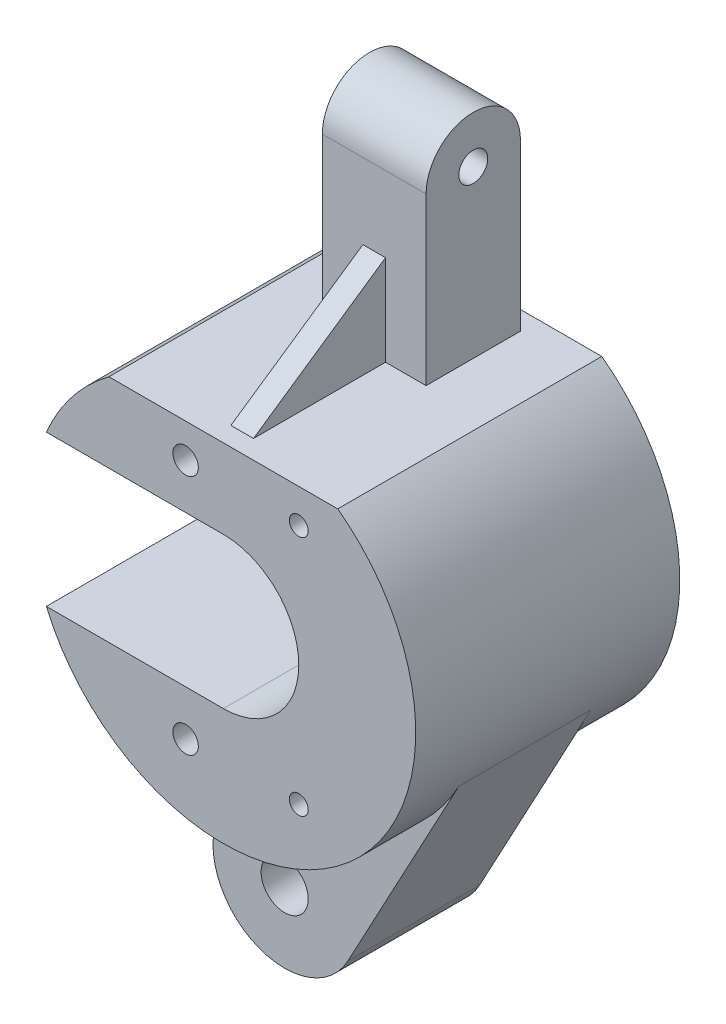
ISO-10303-21;
HEADER;
FILE_DESCRIPTION(('STEP AP214'),'2;1');
FILE_NAME('part.step','',(''),(''),'','','');
FILE_SCHEMA(('AUTOMOTIVE_DESIGN { 1 0 10303 214 1 1 1 1 }'));
ENDSEC;
DATA;
#1=APPLICATION_CONTEXT('core data for automotive mechanical design processes');
#2=APPLICATION_PROTOCOL_DEFINITION('international standard','automotive_design',2000,#1);
#3=PRODUCT_CONTEXT('',#1,'mechanical');
#4=PRODUCT('Part','Part','',(#3));
#5=PRODUCT_RELATED_PRODUCT_CATEGORY('part','',(#4));
#6=PRODUCT_DEFINITION_FORMATION('','',#4);
#7=PRODUCT_DEFINITION_CONTEXT('part definition',#1,'design');
#8=PRODUCT_DEFINITION('design','',#6,#7);
#9=PRODUCT_DEFINITION_SHAPE('','',#8);
#10=(LENGTH_UNIT() NAMED_UNIT(*) SI_UNIT(.MILLI.,.METRE.));
#11=(NAMED_UNIT(*) PLANE_ANGLE_UNIT() SI_UNIT($,.RADIAN.));
#12=(NAMED_UNIT(*) SI_UNIT($,.STERADIAN.) SOLID_ANGLE_UNIT());
#13=UNCERTAINTY_MEASURE_WITH_UNIT(LENGTH_MEASURE(1.E-05),#10,'distance_accuracy_value','');
#14=(GEOMETRIC_REPRESENTATION_CONTEXT(3) GLOBAL_UNCERTAINTY_ASSIGNED_CONTEXT((#13)) GLOBAL_UNIT_ASSIGNED_CONTEXT((#10,
#11,#12)) REPRESENTATION_CONTEXT('',''));
#15=CARTESIAN_POINT('',(0.,0.,0.));
#16=DIRECTION('',(0.,0.,1.));
#17=DIRECTION('',(1.,0.,0.));
#18=AXIS2_PLACEMENT_3D('',#15,#16,#17);
#19=CARTESIAN_POINT('',(0.,0.,70.));
#20=DIRECTION('',(0.,0.,1.));
#21=DIRECTION('',(1.,0.,0.));
#22=AXIS2_PLACEMENT_3D('',#19,#20,#21);
#23=PLANE('',#22);
#24=CARTESIAN_POINT('',(39.9916385221974,-64.,70.));
#25=DIRECTION('',(0.,0.,1.));
#26=DIRECTION('',(-1.,0.,0.));
#27=AXIS2_PLACEMENT_3D('',#24,#25,#26);
#28=CIRCLE('',#27,5.);
#29=CARTESIAN_POINT('',(34.9916385221974,-64.,70.));
#30=VERTEX_POINT('',#29);
#31=EDGE_CURVE('E274',#30,#30,#28,.T.);
#32=ORIENTED_EDGE('',*,*,#31,.F.);
#33=EDGE_LOOP('',(#32));
#34=FACE_BOUND('',#33,.T.);
#35=CARTESIAN_POINT('',(39.9916385221974,64.,70.));
#36=DIRECTION('',(0.,0.,1.));
#37=DIRECTION('',(1.,0.,0.));
#38=AXIS2_PLACEMENT_3D('',#35,#36,#37);
#39=CIRCLE('',#38,5.);
#40=CARTESIAN_POINT('',(44.9916385221974,64.,70.));
#41=VERTEX_POINT('',#40);
#42=EDGE_CURVE('E284',#41,#41,#39,.T.);
#43=ORIENTED_EDGE('',*,*,#42,.F.);
#44=EDGE_LOOP('',(#43));
#45=FACE_BOUND('',#44,.T.);
#46=CARTESIAN_POINT('',(0.,0.,70.));
#47=DIRECTION('',(0.,0.,1.));
#48=DIRECTION('',(1.,0.,0.));
#49=AXIS2_PLACEMENT_3D('',#46,#47,#48);
#50=CIRCLE('',#49,102.);
#51=CARTESIAN_POINT('',(-93.8296328459192,-40.,70.));
#52=VERTEX_POINT('',#51);
#53=CARTESIAN_POINT('',(60.6630035524124,82.,70.));
#54=VERTEX_POINT('',#53);
#55=EDGE_CURVE('E289',#52,#54,#50,.T.);
#56=ORIENTED_EDGE('',*,*,#55,.T.);
#57=DIRECTION('',(-1.,0.,0.));
#58=VECTOR('',#57,1.);
#59=CARTESIAN_POINT('',(-60.6630035524124,82.,70.));
#60=LINE('',#59,#58);
#61=CARTESIAN_POINT('',(-60.6630035524124,82.,70.));
#62=VERTEX_POINT('',#61);
#63=EDGE_CURVE('E291',#54,#62,#60,.T.);
#64=ORIENTED_EDGE('',*,*,#63,.T.);
#65=CARTESIAN_POINT('',(0.,0.,70.));
#66=DIRECTION('',(0.,0.,1.));
#67=DIRECTION('',(1.,0.,0.));
#68=AXIS2_PLACEMENT_3D('',#65,#66,#67);
#69=CIRCLE('',#68,102.);
#70=CARTESIAN_POINT('',(-93.8296328459192,40.,70.));
#71=VERTEX_POINT('',#70);
#72=EDGE_CURVE('E297',#62,#71,#69,.T.);
#73=ORIENTED_EDGE('',*,*,#72,.T.);
#74=DIRECTION('',(1.,0.,0.));
#75=VECTOR('',#74,1.);
#76=CARTESIAN_POINT('',(0.,40.,70.));
#77=LINE('',#76,#75);
#78=CARTESIAN_POINT('',(0.,40.,70.));
#79=VERTEX_POINT('',#78);
#80=EDGE_CURVE('E298',#71,#79,#77,.T.);
#81=ORIENTED_EDGE('',*,*,#80,.T.);
#82=CARTESIAN_POINT('',(0.,0.,70.));
#83=DIRECTION('',(0.,0.,-1.));
#84=DIRECTION('',(1.,0.,0.));
#85=AXIS2_PLACEMENT_3D('',#82,#83,#84);
#86=CIRCLE('',#85,40.);
#87=CARTESIAN_POINT('',(0.,-40.,70.));
#88=VERTEX_POINT('',#87);
#89=EDGE_CURVE('E296',#79,#88,#86,.T.);
#90=ORIENTED_EDGE('',*,*,#89,.T.);
#91=DIRECTION('',(-1.,0.,0.));
#92=VECTOR('',#91,1.);
#93=CARTESIAN_POINT('',(0.,-40.,70.));
#94=LINE('',#93,#92);
#95=EDGE_CURVE('E305',#88,#52,#94,.T.);
#96=ORIENTED_EDGE('',*,*,#95,.T.);
#97=EDGE_LOOP('',(#56,#64,#73,#81,#90,#96));
#98=FACE_BOUND('',#97,.T.);
#99=CARTESIAN_POINT('',(-20.,64.,70.));
#100=DIRECTION('',(0.,0.,1.));
#101=DIRECTION('',(1.,0.,0.));
#102=AXIS2_PLACEMENT_3D('',#99,#100,#101);
#103=CIRCLE('',#102,6.75);
#104=CARTESIAN_POINT('',(-13.25,64.,70.));
#105=VERTEX_POINT('',#104);
#106=EDGE_CURVE('E282',#105,#105,#103,.T.);
#107=ORIENTED_EDGE('',*,*,#106,.F.);
#108=EDGE_LOOP('',(#107));
#109=FACE_BOUND('',#108,.T.);
#110=CARTESIAN_POINT('',(-20.,-64.,70.));
#111=DIRECTION('',(0.,0.,1.));
#112=DIRECTION('',(-1.,0.,0.));
#113=AXIS2_PLACEMENT_3D('',#110,#111,#112);
#114=CIRCLE('',#113,6.75);
#115=CARTESIAN_POINT('',(-26.75,-64.,70.));
#116=VERTEX_POINT('',#115);
#117=EDGE_CURVE('E275',#116,#116,#114,.T.);
#118=ORIENTED_EDGE('',*,*,#117,.F.);
#119=EDGE_LOOP('',(#118));
#120=FACE_BOUND('',#119,.T.);
#121=ADVANCED_FACE('F43',(#34,#45,#98,#109,#120),#23,.T.);
#122=CARTESIAN_POINT('',(0.,0.,-70.));
#123=DIRECTION('',(0.,0.,1.));
#124=DIRECTION('',(1.,0.,0.));
#125=AXIS2_PLACEMENT_3D('',#122,#123,#124);
#126=PLANE('',#125);
#127=CARTESIAN_POINT('',(39.9916385221974,-64.,-70.));
#128=DIRECTION('',(0.,0.,1.));
#129=DIRECTION('',(1.,0.,0.));
#130=AXIS2_PLACEMENT_3D('',#127,#128,#129);
#131=CIRCLE('',#130,7.00000000000006);
#132=CARTESIAN_POINT('',(46.9916385221974,-64.,-70.));
#133=VERTEX_POINT('',#132);
#134=EDGE_CURVE('E337',#133,#133,#131,.T.);
#135=ORIENTED_EDGE('',*,*,#134,.T.);
#136=EDGE_LOOP('',(#135));
#137=FACE_BOUND('',#136,.T.);
#138=CARTESIAN_POINT('',(39.9916385221974,64.,-70.));
#139=DIRECTION('',(0.,0.,1.));
#140=DIRECTION('',(1.,0.,0.));
#141=AXIS2_PLACEMENT_3D('',#138,#139,#140);
#142=CIRCLE('',#141,7.00000000000006);
#143=CARTESIAN_POINT('',(46.9916385221974,64.,-70.));
#144=VERTEX_POINT('',#143);
#145=EDGE_CURVE('E334',#144,#144,#142,.T.);
#146=ORIENTED_EDGE('',*,*,#145,.T.);
#147=EDGE_LOOP('',(#146));
#148=FACE_BOUND('',#147,.T.);
#149=CARTESIAN_POINT('',(0.,0.,-70.));
#150=DIRECTION('',(0.,0.,1.));
#151=DIRECTION('',(1.,0.,0.));
#152=AXIS2_PLACEMENT_3D('',#149,#150,#151);
#153=CIRCLE('',#152,102.);
#154=CARTESIAN_POINT('',(-93.8296328459192,-40.,-70.));
#155=VERTEX_POINT('',#154);
#156=CARTESIAN_POINT('',(60.6630035524124,82.,-70.));
#157=VERTEX_POINT('',#156);
#158=EDGE_CURVE('E287',#155,#157,#153,.T.);
#159=ORIENTED_EDGE('',*,*,#158,.F.);
#160=DIRECTION('',(-1.,0.,0.));
#161=VECTOR('',#160,1.);
#162=CARTESIAN_POINT('',(0.,-40.,-70.));
#163=LINE('',#162,#161);
#164=CARTESIAN_POINT('',(0.,-40.,-70.));
#165=VERTEX_POINT('',#164);
#166=EDGE_CURVE('E294',#165,#155,#163,.T.);
#167=ORIENTED_EDGE('',*,*,#166,.F.);
#168=CARTESIAN_POINT('',(0.,0.,-70.));
#169=DIRECTION('',(0.,0.,-1.));
#170=DIRECTION('',(1.,0.,0.));
#171=AXIS2_PLACEMENT_3D('',#168,#169,#170);
#172=CIRCLE('',#171,40.);
#173=CARTESIAN_POINT('',(0.,40.,-70.));
#174=VERTEX_POINT('',#173);
#175=EDGE_CURVE('E311',#174,#165,#172,.T.);
#176=ORIENTED_EDGE('',*,*,#175,.F.);
#177=DIRECTION('',(1.,0.,0.));
#178=VECTOR('',#177,1.);
#179=CARTESIAN_POINT('',(0.,40.,-70.));
#180=LINE('',#179,#178);
#181=CARTESIAN_POINT('',(-93.8296328459192,40.,-70.));
#182=VERTEX_POINT('',#181);
#183=EDGE_CURVE('E313',#182,#174,#180,.T.);
#184=ORIENTED_EDGE('',*,*,#183,.F.);
#185=CARTESIAN_POINT('',(0.,0.,-70.));
#186=DIRECTION('',(0.,0.,1.));
#187=DIRECTION('',(1.,0.,0.));
#188=AXIS2_PLACEMENT_3D('',#185,#186,#187);
#189=CIRCLE('',#188,102.);
#190=CARTESIAN_POINT('',(-60.6630035524124,82.,-70.));
#191=VERTEX_POINT('',#190);
#192=EDGE_CURVE('E310',#191,#182,#189,.T.);
#193=ORIENTED_EDGE('',*,*,#192,.F.);
#194=DIRECTION('',(-1.,0.,0.));
#195=VECTOR('',#194,1.);
#196=CARTESIAN_POINT('',(-60.6630035524124,82.,-70.));
#197=LINE('',#196,#195);
#198=EDGE_CURVE('E307',#157,#191,#197,.T.);
#199=ORIENTED_EDGE('',*,*,#198,.F.);
#200=EDGE_LOOP('',(#159,#167,#176,#184,#193,#199));
#201=FACE_BOUND('',#200,.T.);
#202=CARTESIAN_POINT('',(-20.,64.,-70.));
#203=DIRECTION('',(0.,0.,1.));
#204=DIRECTION('',(1.,0.,0.));
#205=AXIS2_PLACEMENT_3D('',#202,#203,#204);
#206=CIRCLE('',#205,6.75);
#207=CARTESIAN_POINT('',(-13.25,64.,-70.));
#208=VERTEX_POINT('',#207);
#209=EDGE_CURVE('E278',#208,#208,#206,.T.);
#210=ORIENTED_EDGE('',*,*,#209,.T.);
#211=EDGE_LOOP('',(#210));
#212=FACE_BOUND('',#211,.T.);
#213=CARTESIAN_POINT('',(-20.,-64.,-70.));
#214=DIRECTION('',(0.,0.,1.));
#215=DIRECTION('',(-1.,0.,0.));
#216=AXIS2_PLACEMENT_3D('',#213,#214,#215);
#217=CIRCLE('',#216,6.75);
#218=CARTESIAN_POINT('',(-26.75,-64.,-70.));
#219=VERTEX_POINT('',#218);
#220=EDGE_CURVE('E271',#219,#219,#217,.T.);
#221=ORIENTED_EDGE('',*,*,#220,.T.);
#222=EDGE_LOOP('',(#221));
#223=FACE_BOUND('',#222,.T.);
#224=ADVANCED_FACE('F348',(#137,#148,#201,#212,#223),#126,.F.);
#225=CARTESIAN_POINT('',(0.,0.,70.));
#226=DIRECTION('',(0.,0.,-1.));
#227=DIRECTION('',(-1.,0.,0.));
#228=AXIS2_PLACEMENT_3D('',#225,#226,#227);
#229=CYLINDRICAL_SURFACE('',#228,102.);
#230=DIRECTION('',(0.,0.,-1.));
#231=VECTOR('',#230,1.);
#232=CARTESIAN_POINT('',(-27.5,-98.2229606558466,35.));
#233=LINE('',#232,#231);
#234=CARTESIAN_POINT('',(-27.5,-98.2229606558466,35.));
#235=VERTEX_POINT('',#234);
#236=CARTESIAN_POINT('',(-27.5,-98.2229606558466,-35.));
#237=VERTEX_POINT('',#236);
#238=EDGE_CURVE('E64',#235,#237,#233,.T.);
#239=ORIENTED_EDGE('',*,*,#238,.F.);
#240=CARTESIAN_POINT('',(0.,0.,35.));
#241=DIRECTION('',(0.,0.,1.));
#242=DIRECTION('',(1.,0.,0.));
#243=AXIS2_PLACEMENT_3D('',#240,#241,#242);
#244=CIRCLE('',#243,102.);
#245=CARTESIAN_POINT('',(-2.49082671878777,-101.969582632553,35.));
#246=VERTEX_POINT('',#245);
#247=EDGE_CURVE('E56',#235,#246,#244,.T.);
#248=ORIENTED_EDGE('',*,*,#247,.T.);
#249=DIRECTION('',(0.,0.,-1.));
#250=VECTOR('',#249,1.);
#251=CARTESIAN_POINT('',(-2.49082671878777,-101.969582632553,35.));
#252=LINE('',#251,#250);
#253=CARTESIAN_POINT('',(-2.49082671878777,-101.969582632553,-35.));
#254=VERTEX_POINT('',#253);
#255=EDGE_CURVE('E201',#246,#254,#252,.T.);
#256=ORIENTED_EDGE('',*,*,#255,.T.);
#257=CARTESIAN_POINT('',(0.,0.,-35.));
#258=DIRECTION('',(0.,0.,1.));
#259=DIRECTION('',(1.,0.,0.));
#260=AXIS2_PLACEMENT_3D('',#257,#258,#259);
#261=CIRCLE('',#260,102.);
#262=EDGE_CURVE('E705',#237,#254,#261,.T.);
#263=ORIENTED_EDGE('',*,*,#262,.F.);
#264=EDGE_LOOP('',(#239,#248,#256,#263));
#265=FACE_BOUND('',#264,.T.);
#266=DIRECTION('',(0.,0.,-1.));
#267=VECTOR('',#266,1.);
#268=CARTESIAN_POINT('',(-1.81474518083109,-101.983855094464,35.));
#269=LINE('',#268,#267);
#270=CARTESIAN_POINT('',(-1.81474518083109,-101.983855094464,35.));
#271=VERTEX_POINT('',#270);
#272=CARTESIAN_POINT('',(-1.81474518083109,-101.983855094464,-35.));
#273=VERTEX_POINT('',#272);
#274=EDGE_CURVE('E424',#271,#273,#269,.T.);
#275=ORIENTED_EDGE('',*,*,#274,.F.);
#276=CARTESIAN_POINT('',(89.8741576873943,-48.2352130707575,35.));
#277=VERTEX_POINT('',#276);
#278=EDGE_CURVE('E725',#271,#277,#244,.T.);
#279=ORIENTED_EDGE('',*,*,#278,.T.);
#280=DIRECTION('',(0.,0.,-1.));
#281=VECTOR('',#280,1.);
#282=CARTESIAN_POINT('',(89.8741576873943,-48.2352130707575,35.));
#283=LINE('',#282,#281);
#284=CARTESIAN_POINT('',(89.8741576873943,-48.2352130707575,-35.));
#285=VERTEX_POINT('',#284);
#286=EDGE_CURVE('E202',#277,#285,#283,.T.);
#287=ORIENTED_EDGE('',*,*,#286,.T.);
#288=EDGE_CURVE('E704',#273,#285,#261,.T.);
#289=ORIENTED_EDGE('',*,*,#288,.F.);
#290=EDGE_LOOP('',(#275,#279,#287,#289));
#291=FACE_BOUND('',#290,.T.);
#292=ORIENTED_EDGE('',*,*,#158,.T.);
#293=DIRECTION('',(0.,0.,-1.));
#294=VECTOR('',#293,1.);
#295=CARTESIAN_POINT('',(60.6630035524124,82.,70.));
#296=LINE('',#295,#294);
#297=EDGE_CURVE('E329',#54,#157,#296,.T.);
#298=ORIENTED_EDGE('',*,*,#297,.F.);
#299=ORIENTED_EDGE('',*,*,#55,.F.);
#300=DIRECTION('',(0.,0.,-1.));
#301=VECTOR('',#300,1.);
#302=CARTESIAN_POINT('',(-93.8296328459192,-40.,70.));
#303=LINE('',#302,#301);
#304=EDGE_CURVE('E302',#52,#155,#303,.T.);
#305=ORIENTED_EDGE('',*,*,#304,.T.);
#306=EDGE_LOOP('',(#292,#298,#299,#305));
#307=FACE_BOUND('',#306,.T.);
#308=ADVANCED_FACE('F353',(#265,#291,#307),#229,.T.);
#309=CARTESIAN_POINT('',(-60.6630035524124,82.,70.));
#310=DIRECTION('',(0.,-1.,0.));
#311=DIRECTION('',(0.,0.,-1.));
#312=AXIS2_PLACEMENT_3D('',#309,#310,#311);
#313=PLANE('',#312);
#314=DIRECTION('',(-1.,0.,0.));
#315=VECTOR('',#314,1.);
#316=CARTESIAN_POINT('',(27.5,82.,-10.));
#317=LINE('',#316,#315);
#318=CARTESIAN_POINT('',(27.5,82.,-10.));
#319=VERTEX_POINT('',#318);
#320=CARTESIAN_POINT('',(6.,82.,-10.));
#321=VERTEX_POINT('',#320);
#322=EDGE_CURVE('E268',#319,#321,#317,.T.);
#323=ORIENTED_EDGE('',*,*,#322,.T.);
#324=DIRECTION('',(0.,0.,-1.));
#325=VECTOR('',#324,1.);
#326=CARTESIAN_POINT('',(6.,82.,0.));
#327=LINE('',#326,#325);
#328=CARTESIAN_POINT('',(6.00000000000001,82.,60.));
#329=VERTEX_POINT('',#328);
#330=EDGE_CURVE('E220',#329,#321,#327,.T.);
#331=ORIENTED_EDGE('',*,*,#330,.F.);
#332=DIRECTION('',(-1.,0.,0.));
#333=VECTOR('',#332,1.);
#334=CARTESIAN_POINT('',(6.,82.,60.));
#335=LINE('',#334,#333);
#336=CARTESIAN_POINT('',(-6.,82.,60.));
#337=VERTEX_POINT('',#336);
#338=EDGE_CURVE('E219',#329,#337,#335,.T.);
#339=ORIENTED_EDGE('',*,*,#338,.T.);
#340=DIRECTION('',(0.,0.,-1.));
#341=VECTOR('',#340,1.);
#342=CARTESIAN_POINT('',(-6.,82.,0.));
#343=LINE('',#342,#341);
#344=CARTESIAN_POINT('',(-6.,82.,-10.));
#345=VERTEX_POINT('',#344);
#346=EDGE_CURVE('E212',#337,#345,#343,.T.);
#347=ORIENTED_EDGE('',*,*,#346,.T.);
#348=CARTESIAN_POINT('',(-27.5,82.,-10.));
#349=VERTEX_POINT('',#348);
#350=EDGE_CURVE('E270',#345,#349,#317,.T.);
#351=ORIENTED_EDGE('',*,*,#350,.T.);
#352=DIRECTION('',(0.,0.,-1.));
#353=VECTOR('',#352,1.);
#354=CARTESIAN_POINT('',(-27.5,82.,0.));
#355=LINE('',#354,#353);
#356=CARTESIAN_POINT('',(-27.5,82.,-60.));
#357=VERTEX_POINT('',#356);
#358=EDGE_CURVE('E253',#349,#357,#355,.T.);
#359=ORIENTED_EDGE('',*,*,#358,.T.);
#360=DIRECTION('',(-1.,0.,0.));
#361=VECTOR('',#360,1.);
#362=CARTESIAN_POINT('',(27.5,82.,-60.));
#363=LINE('',#362,#361);
#364=CARTESIAN_POINT('',(27.5,82.,-60.));
#365=VERTEX_POINT('',#364);
#366=EDGE_CURVE('E262',#365,#357,#363,.T.);
#367=ORIENTED_EDGE('',*,*,#366,.F.);
#368=DIRECTION('',(0.,0.,-1.));
#369=VECTOR('',#368,1.);
#370=CARTESIAN_POINT('',(27.5,82.,0.));
#371=LINE('',#370,#369);
#372=EDGE_CURVE('E237',#319,#365,#371,.T.);
#373=ORIENTED_EDGE('',*,*,#372,.F.);
#374=EDGE_LOOP('',(#323,#331,#339,#347,#351,#359,#367,#373));
#375=FACE_BOUND('',#374,.T.);
#376=ORIENTED_EDGE('',*,*,#198,.T.);
#377=DIRECTION('',(0.,0.,-1.));
#378=VECTOR('',#377,1.);
#379=CARTESIAN_POINT('',(-60.6630035524124,82.,70.));
#380=LINE('',#379,#378);
#381=EDGE_CURVE('E330',#62,#191,#380,.T.);
#382=ORIENTED_EDGE('',*,*,#381,.F.);
#383=ORIENTED_EDGE('',*,*,#63,.F.);
#384=ORIENTED_EDGE('',*,*,#297,.T.);
#385=EDGE_LOOP('',(#376,#382,#383,#384));
#386=FACE_BOUND('',#385,.T.);
#387=ADVANCED_FACE('F407',(#375,#386),#313,.F.);
#388=CARTESIAN_POINT('',(0.,0.,70.));
#389=DIRECTION('',(0.,0.,-1.));
#390=DIRECTION('',(-1.,0.,0.));
#391=AXIS2_PLACEMENT_3D('',#388,#389,#390);
#392=CYLINDRICAL_SURFACE('',#391,102.);
#393=ORIENTED_EDGE('',*,*,#192,.T.);
#394=DIRECTION('',(0.,0.,-1.));
#395=VECTOR('',#394,1.);
#396=CARTESIAN_POINT('',(-93.8296328459192,40.,70.));
#397=LINE('',#396,#395);
#398=EDGE_CURVE('E322',#71,#182,#397,.T.);
#399=ORIENTED_EDGE('',*,*,#398,.F.);
#400=ORIENTED_EDGE('',*,*,#72,.F.);
#401=ORIENTED_EDGE('',*,*,#381,.T.);
#402=EDGE_LOOP('',(#393,#399,#400,#401));
#403=FACE_BOUND('',#402,.T.);
#404=ADVANCED_FACE('F401',(#403),#392,.T.);
#405=CARTESIAN_POINT('',(0.,40.,70.));
#406=DIRECTION('',(0.,1.,0.));
#407=DIRECTION('',(-1.,0.,0.));
#408=AXIS2_PLACEMENT_3D('',#405,#406,#407);
#409=PLANE('',#408);
#410=ORIENTED_EDGE('',*,*,#183,.T.);
#411=DIRECTION('',(0.,0.,-1.));
#412=VECTOR('',#411,1.);
#413=CARTESIAN_POINT('',(0.,40.,70.));
#414=LINE('',#413,#412);
#415=EDGE_CURVE('E321',#79,#174,#414,.T.);
#416=ORIENTED_EDGE('',*,*,#415,.F.);
#417=ORIENTED_EDGE('',*,*,#80,.F.);
#418=ORIENTED_EDGE('',*,*,#398,.T.);
#419=EDGE_LOOP('',(#410,#416,#417,#418));
#420=FACE_BOUND('',#419,.T.);
#421=ADVANCED_FACE('F397',(#420),#409,.F.);
#422=CARTESIAN_POINT('',(0.,0.,70.));
#423=DIRECTION('',(0.,0.,-1.));
#424=DIRECTION('',(-1.,0.,0.));
#425=AXIS2_PLACEMENT_3D('',#422,#423,#424);
#426=CYLINDRICAL_SURFACE('',#425,40.);
#427=ORIENTED_EDGE('',*,*,#175,.T.);
#428=DIRECTION('',(0.,0.,-1.));
#429=VECTOR('',#428,1.);
#430=CARTESIAN_POINT('',(0.,-40.,70.));
#431=LINE('',#430,#429);
#432=EDGE_CURVE('E318',#88,#165,#431,.T.);
#433=ORIENTED_EDGE('',*,*,#432,.F.);
#434=ORIENTED_EDGE('',*,*,#89,.F.);
#435=ORIENTED_EDGE('',*,*,#415,.T.);
#436=EDGE_LOOP('',(#427,#433,#434,#435));
#437=FACE_BOUND('',#436,.T.);
#438=ADVANCED_FACE('F391',(#437),#426,.F.);
#439=CARTESIAN_POINT('',(0.,-40.,70.));
#440=DIRECTION('',(0.,-1.,0.));
#441=DIRECTION('',(1.,0.,0.));
#442=AXIS2_PLACEMENT_3D('',#439,#440,#441);
#443=PLANE('',#442);
#444=ORIENTED_EDGE('',*,*,#166,.T.);
#445=ORIENTED_EDGE('',*,*,#304,.F.);
#446=ORIENTED_EDGE('',*,*,#95,.F.);
#447=ORIENTED_EDGE('',*,*,#432,.T.);
#448=EDGE_LOOP('',(#444,#445,#446,#447));
#449=FACE_BOUND('',#448,.T.);
#450=ADVANCED_FACE('F395',(#449),#443,.F.);
#451=CARTESIAN_POINT('',(39.9916385221974,64.,70.));
#452=DIRECTION('',(0.,0.,-1.));
#453=DIRECTION('',(-1.,0.,0.));
#454=AXIS2_PLACEMENT_3D('',#451,#452,#453);
#455=CYLINDRICAL_SURFACE('',#454,5.);
#456=CARTESIAN_POINT('',(39.9916385221974,64.,-67.9999999999999));
#457=DIRECTION('',(0.,0.,1.));
#458=DIRECTION('',(1.,0.,0.));
#459=AXIS2_PLACEMENT_3D('',#456,#457,#458);
#460=CIRCLE('',#459,5.);
#461=CARTESIAN_POINT('',(44.9916385221974,64.,-67.9999999999999));
#462=VERTEX_POINT('',#461);
#463=EDGE_CURVE('E11',#462,#462,#460,.F.);
#464=ORIENTED_EDGE('',*,*,#463,.T.);
#465=EDGE_LOOP('',(#464));
#466=FACE_BOUND('',#465,.T.);
#467=ORIENTED_EDGE('',*,*,#42,.T.);
#468=EDGE_LOOP('',(#467));
#469=FACE_BOUND('',#468,.T.);
#470=ADVANCED_FACE('F386',(#466,#469),#455,.F.);
#471=CARTESIAN_POINT('',(-20.,64.,70.));
#472=DIRECTION('',(0.,0.,-1.));
#473=DIRECTION('',(-1.,0.,0.));
#474=AXIS2_PLACEMENT_3D('',#471,#472,#473);
#475=CYLINDRICAL_SURFACE('',#474,6.75);
#476=ORIENTED_EDGE('',*,*,#106,.T.);
#477=EDGE_LOOP('',(#476));
#478=FACE_BOUND('',#477,.T.);
#479=ORIENTED_EDGE('',*,*,#209,.F.);
#480=EDGE_LOOP('',(#479));
#481=FACE_BOUND('',#480,.T.);
#482=ADVANCED_FACE('F378',(#478,#481),#475,.F.);
#483=CARTESIAN_POINT('',(39.9916385221974,-64.,70.));
#484=DIRECTION('',(0.,0.,-1.));
#485=DIRECTION('',(-1.,0.,0.));
#486=AXIS2_PLACEMENT_3D('',#483,#484,#485);
#487=CYLINDRICAL_SURFACE('',#486,5.);
#488=CARTESIAN_POINT('',(39.9916385221974,-64.,-67.9999999999999));
#489=DIRECTION('',(0.,0.,1.));
#490=DIRECTION('',(1.,0.,0.));
#491=AXIS2_PLACEMENT_3D('',#488,#489,#490);
#492=CIRCLE('',#491,5.);
#493=CARTESIAN_POINT('',(44.9916385221974,-64.,-67.9999999999999));
#494=VERTEX_POINT('',#493);
#495=EDGE_CURVE('E55',#494,#494,#492,.F.);
#496=ORIENTED_EDGE('',*,*,#495,.T.);
#497=EDGE_LOOP('',(#496));
#498=FACE_BOUND('',#497,.T.);
#499=ORIENTED_EDGE('',*,*,#31,.T.);
#500=EDGE_LOOP('',(#499));
#501=FACE_BOUND('',#500,.T.);
#502=ADVANCED_FACE('F341',(#498,#501),#487,.F.);
#503=CARTESIAN_POINT('',(-20.,-64.,70.));
#504=DIRECTION('',(0.,0.,-1.));
#505=DIRECTION('',(-1.,0.,0.));
#506=AXIS2_PLACEMENT_3D('',#503,#504,#505);
#507=CYLINDRICAL_SURFACE('',#506,6.75);
#508=ORIENTED_EDGE('',*,*,#117,.T.);
#509=EDGE_LOOP('',(#508));
#510=FACE_BOUND('',#509,.T.);
#511=ORIENTED_EDGE('',*,*,#220,.F.);
#512=EDGE_LOOP('',(#511));
#513=FACE_BOUND('',#512,.T.);
#514=ADVANCED_FACE('F365',(#510,#513),#507,.F.);
#515=CARTESIAN_POINT('',(27.5,0.,-10.));
#516=DIRECTION('',(0.,0.,-1.));
#517=DIRECTION('',(-1.,0.,0.));
#518=AXIS2_PLACEMENT_3D('',#515,#516,#517);
#519=PLANE('',#518);
#520=DIRECTION('',(-1.,0.,0.));
#521=VECTOR('',#520,1.);
#522=CARTESIAN_POINT('',(6.,130.,-10.));
#523=LINE('',#522,#521);
#524=CARTESIAN_POINT('',(6.,130.,-10.));
#525=VERTEX_POINT('',#524);
#526=CARTESIAN_POINT('',(-6.,130.,-10.));
#527=VERTEX_POINT('',#526);
#528=EDGE_CURVE('E229',#525,#527,#523,.T.);
#529=ORIENTED_EDGE('',*,*,#528,.F.);
#530=DIRECTION('',(0.,-1.,0.));
#531=VECTOR('',#530,1.);
#532=CARTESIAN_POINT('',(6.,0.,-10.));
#533=LINE('',#532,#531);
#534=EDGE_CURVE('E211',#525,#321,#533,.T.);
#535=ORIENTED_EDGE('',*,*,#534,.T.);
#536=ORIENTED_EDGE('',*,*,#322,.F.);
#537=DIRECTION('',(0.,-1.,0.));
#538=VECTOR('',#537,1.);
#539=CARTESIAN_POINT('',(27.5,0.,-10.));
#540=LINE('',#539,#538);
#541=CARTESIAN_POINT('',(27.5,170.,-10.));
#542=VERTEX_POINT('',#541);
#543=EDGE_CURVE('E233',#542,#319,#540,.T.);
#544=ORIENTED_EDGE('',*,*,#543,.F.);
#545=DIRECTION('',(-1.,0.,0.));
#546=VECTOR('',#545,1.);
#547=CARTESIAN_POINT('',(27.5,170.,-10.));
#548=LINE('',#547,#546);
#549=CARTESIAN_POINT('',(-27.5,170.,-10.));
#550=VERTEX_POINT('',#549);
#551=EDGE_CURVE('E248',#542,#550,#548,.T.);
#552=ORIENTED_EDGE('',*,*,#551,.T.);
#553=DIRECTION('',(0.,-1.,0.));
#554=VECTOR('',#553,1.);
#555=CARTESIAN_POINT('',(-27.5,0.,-10.));
#556=LINE('',#555,#554);
#557=EDGE_CURVE('E235',#550,#349,#556,.T.);
#558=ORIENTED_EDGE('',*,*,#557,.T.);
#559=ORIENTED_EDGE('',*,*,#350,.F.);
#560=DIRECTION('',(0.,-1.,0.));
#561=VECTOR('',#560,1.);
#562=CARTESIAN_POINT('',(-6.,0.,-10.));
#563=LINE('',#562,#561);
#564=EDGE_CURVE('E209',#527,#345,#563,.T.);
#565=ORIENTED_EDGE('',*,*,#564,.F.);
#566=EDGE_LOOP('',(#529,#535,#536,#544,#552,#558,#559,#565));
#567=FACE_BOUND('',#566,.T.);
#568=ADVANCED_FACE('F368',(#567),#519,.F.);
#569=CARTESIAN_POINT('',(27.5,0.,-60.));
#570=DIRECTION('',(0.,0.,-1.));
#571=DIRECTION('',(-1.,0.,0.));
#572=AXIS2_PLACEMENT_3D('',#569,#570,#571);
#573=PLANE('',#572);
#574=DIRECTION('',(0.,-1.,0.));
#575=VECTOR('',#574,1.);
#576=CARTESIAN_POINT('',(-27.5,0.,-60.));
#577=LINE('',#576,#575);
#578=CARTESIAN_POINT('',(-27.5,170.,-60.));
#579=VERTEX_POINT('',#578);
#580=EDGE_CURVE('E251',#579,#357,#577,.T.);
#581=ORIENTED_EDGE('',*,*,#580,.F.);
#582=DIRECTION('',(-1.,0.,0.));
#583=VECTOR('',#582,1.);
#584=CARTESIAN_POINT('',(27.5,170.,-60.));
#585=LINE('',#584,#583);
#586=CARTESIAN_POINT('',(27.5,170.,-60.));
#587=VERTEX_POINT('',#586);
#588=EDGE_CURVE('E265',#587,#579,#585,.T.);
#589=ORIENTED_EDGE('',*,*,#588,.F.);
#590=DIRECTION('',(0.,-1.,0.));
#591=VECTOR('',#590,1.);
#592=CARTESIAN_POINT('',(27.5,0.,-60.));
#593=LINE('',#592,#591);
#594=EDGE_CURVE('E238',#587,#365,#593,.T.);
#595=ORIENTED_EDGE('',*,*,#594,.T.);
#596=ORIENTED_EDGE('',*,*,#366,.T.);
#597=EDGE_LOOP('',(#581,#589,#595,#596));
#598=FACE_BOUND('',#597,.T.);
#599=ADVANCED_FACE('F372',(#598),#573,.T.);
#600=CARTESIAN_POINT('',(27.5,170.,-35.));
#601=DIRECTION('',(-1.,0.,0.));
#602=DIRECTION('',(0.,0.,1.));
#603=AXIS2_PLACEMENT_3D('',#600,#601,#602);
#604=CYLINDRICAL_SURFACE('',#603,25.);
#605=CARTESIAN_POINT('',(-27.5,170.,-35.));
#606=DIRECTION('',(1.,0.,0.));
#607=DIRECTION('',(0.,0.,-1.));
#608=AXIS2_PLACEMENT_3D('',#605,#606,#607);
#609=CIRCLE('',#608,25.);
#610=EDGE_CURVE('E258',#579,#550,#609,.T.);
#611=ORIENTED_EDGE('',*,*,#610,.T.);
#612=ORIENTED_EDGE('',*,*,#551,.F.);
#613=CARTESIAN_POINT('',(27.5,170.,-35.));
#614=DIRECTION('',(1.,0.,0.));
#615=DIRECTION('',(0.,0.,-1.));
#616=AXIS2_PLACEMENT_3D('',#613,#614,#615);
#617=CIRCLE('',#616,25.);
#618=EDGE_CURVE('E243',#587,#542,#617,.T.);
#619=ORIENTED_EDGE('',*,*,#618,.F.);
#620=ORIENTED_EDGE('',*,*,#588,.T.);
#621=EDGE_LOOP('',(#611,#612,#619,#620));
#622=FACE_BOUND('',#621,.T.);
#623=ADVANCED_FACE('F497',(#622),#604,.T.);
#624=CARTESIAN_POINT('',(27.5,170.,-35.));
#625=DIRECTION('',(-1.,0.,0.));
#626=DIRECTION('',(0.,0.,1.));
#627=AXIS2_PLACEMENT_3D('',#624,#625,#626);
#628=CYLINDRICAL_SURFACE('',#627,7.66897657766724);
#629=CARTESIAN_POINT('',(27.5,170.,-35.));
#630=DIRECTION('',(1.,0.,0.));
#631=DIRECTION('',(0.,0.,-1.));
#632=AXIS2_PLACEMENT_3D('',#629,#630,#631);
#633=CIRCLE('',#632,7.66897657766724);
#634=CARTESIAN_POINT('',(27.5,170.,-42.6689765776672));
#635=VERTEX_POINT('',#634);
#636=EDGE_CURVE('E241',#635,#635,#633,.T.);
#637=ORIENTED_EDGE('',*,*,#636,.T.);
#638=EDGE_LOOP('',(#637));
#639=FACE_BOUND('',#638,.T.);
#640=CARTESIAN_POINT('',(-27.5,170.,-35.));
#641=DIRECTION('',(1.,0.,0.));
#642=DIRECTION('',(0.,0.,-1.));
#643=AXIS2_PLACEMENT_3D('',#640,#641,#642);
#644=CIRCLE('',#643,7.66897657766724);
#645=CARTESIAN_POINT('',(-27.5,170.,-42.6689765776672));
#646=VERTEX_POINT('',#645);
#647=EDGE_CURVE('E240',#646,#646,#644,.T.);
#648=ORIENTED_EDGE('',*,*,#647,.F.);
#649=EDGE_LOOP('',(#648));
#650=FACE_BOUND('',#649,.T.);
#651=ADVANCED_FACE('F506',(#639,#650),#628,.F.);
#652=CARTESIAN_POINT('',(27.5,0.,0.));
#653=DIRECTION('',(1.,0.,0.));
#654=DIRECTION('',(0.,0.,-1.));
#655=AXIS2_PLACEMENT_3D('',#652,#653,#654);
#656=PLANE('',#655);
#657=ORIENTED_EDGE('',*,*,#543,.T.);
#658=ORIENTED_EDGE('',*,*,#372,.T.);
#659=ORIENTED_EDGE('',*,*,#594,.F.);
#660=ORIENTED_EDGE('',*,*,#618,.T.);
#661=EDGE_LOOP('',(#657,#658,#659,#660));
#662=FACE_BOUND('',#661,.T.);
#663=ORIENTED_EDGE('',*,*,#636,.F.);
#664=EDGE_LOOP('',(#663));
#665=FACE_BOUND('',#664,.T.);
#666=ADVANCED_FACE('F517',(#662,#665),#656,.T.);
#667=CARTESIAN_POINT('',(-27.5,0.,0.));
#668=DIRECTION('',(1.,0.,0.));
#669=DIRECTION('',(0.,0.,-1.));
#670=AXIS2_PLACEMENT_3D('',#667,#668,#669);
#671=PLANE('',#670);
#672=ORIENTED_EDGE('',*,*,#557,.F.);
#673=ORIENTED_EDGE('',*,*,#610,.F.);
#674=ORIENTED_EDGE('',*,*,#580,.T.);
#675=ORIENTED_EDGE('',*,*,#358,.F.);
#676=EDGE_LOOP('',(#672,#673,#674,#675));
#677=FACE_BOUND('',#676,.T.);
#678=ORIENTED_EDGE('',*,*,#647,.T.);
#679=EDGE_LOOP('',(#678));
#680=FACE_BOUND('',#679,.T.);
#681=ADVANCED_FACE('F528',(#677,#680),#671,.F.);
#682=CARTESIAN_POINT('',(6.,83.7590227651305,57.434758467518));
#683=DIRECTION('',(0.,-0.824728851845978,-0.565528355551528));
#684=DIRECTION('',(0.,0.565528355551528,-0.824728851845978));
#685=AXIS2_PLACEMENT_3D('',#682,#683,#684);
#686=PLANE('',#685);
#687=DIRECTION('',(0.,-0.565528355551528,0.824728851845978));
#688=VECTOR('',#687,1.);
#689=CARTESIAN_POINT('',(-6.,83.7590227651305,57.434758467518));
#690=LINE('',#689,#688);
#691=EDGE_CURVE('E224',#527,#337,#690,.T.);
#692=ORIENTED_EDGE('',*,*,#691,.T.);
#693=ORIENTED_EDGE('',*,*,#338,.F.);
#694=DIRECTION('',(0.,-0.565528355551528,0.824728851845978));
#695=VECTOR('',#694,1.);
#696=CARTESIAN_POINT('',(6.,83.7590227651305,57.434758467518));
#697=LINE('',#696,#695);
#698=EDGE_CURVE('E213',#525,#329,#697,.T.);
#699=ORIENTED_EDGE('',*,*,#698,.F.);
#700=ORIENTED_EDGE('',*,*,#528,.T.);
#701=EDGE_LOOP('',(#692,#693,#699,#700));
#702=FACE_BOUND('',#701,.T.);
#703=ADVANCED_FACE('F536',(#702),#686,.F.);
#704=CARTESIAN_POINT('',(6.,0.,0.));
#705=DIRECTION('',(1.,0.,0.));
#706=DIRECTION('',(0.,0.,-1.));
#707=AXIS2_PLACEMENT_3D('',#704,#705,#706);
#708=PLANE('',#707);
#709=ORIENTED_EDGE('',*,*,#534,.F.);
#710=ORIENTED_EDGE('',*,*,#698,.T.);
#711=ORIENTED_EDGE('',*,*,#330,.T.);
#712=EDGE_LOOP('',(#709,#710,#711));
#713=FACE_BOUND('',#712,.T.);
#714=ADVANCED_FACE('F544',(#713),#708,.T.);
#715=CARTESIAN_POINT('',(-6.,0.,0.));
#716=DIRECTION('',(1.,0.,0.));
#717=DIRECTION('',(0.,0.,-1.));
#718=AXIS2_PLACEMENT_3D('',#715,#716,#717);
#719=PLANE('',#718);
#720=ORIENTED_EDGE('',*,*,#564,.T.);
#721=ORIENTED_EDGE('',*,*,#346,.F.);
#722=ORIENTED_EDGE('',*,*,#691,.F.);
#723=EDGE_LOOP('',(#720,#721,#722));
#724=FACE_BOUND('',#723,.T.);
#725=ADVANCED_FACE('F553',(#724),#719,.F.);
#726=CARTESIAN_POINT('',(-2.49082671878777,0.,35.));
#727=DIRECTION('',(1.,0.,0.));
#728=DIRECTION('',(0.,0.,-1.));
#729=AXIS2_PLACEMENT_3D('',#726,#727,#728);
#730=PLANE('',#729);
#731=DIRECTION('',(0.,-1.,0.));
#732=VECTOR('',#731,1.);
#733=CARTESIAN_POINT('',(-2.49082671878777,0.,-35.));
#734=LINE('',#733,#732);
#735=CARTESIAN_POINT('',(-2.49082671878776,-101.977840325735,-35.));
#736=VERTEX_POINT('',#735);
#737=EDGE_CURVE('E696',#254,#736,#734,.T.);
#738=ORIENTED_EDGE('',*,*,#737,.F.);
#739=ORIENTED_EDGE('',*,*,#255,.F.);
#740=DIRECTION('',(0.,-1.,0.));
#741=VECTOR('',#740,1.);
#742=CARTESIAN_POINT('',(-2.49082671878777,0.,35.));
#743=LINE('',#742,#741);
#744=CARTESIAN_POINT('',(-2.49082671878776,-101.977840325735,35.));
#745=VERTEX_POINT('',#744);
#746=EDGE_CURVE('E730',#246,#745,#743,.T.);
#747=ORIENTED_EDGE('',*,*,#746,.T.);
#748=DIRECTION('',(0.,0.,-1.));
#749=VECTOR('',#748,1.);
#750=CARTESIAN_POINT('',(-2.49082671878776,-101.977840325735,35.));
#751=LINE('',#750,#749);
#752=EDGE_CURVE('E720',#745,#736,#751,.T.);
#753=ORIENTED_EDGE('',*,*,#752,.T.);
#754=EDGE_LOOP('',(#738,#739,#747,#753));
#755=FACE_BOUND('',#754,.T.);
#756=ADVANCED_FACE('F562',(#755),#730,.T.);
#757=CARTESIAN_POINT('',(-27.5,0.,35.));
#758=DIRECTION('',(1.,0.,0.));
#759=DIRECTION('',(0.,0.,-1.));
#760=AXIS2_PLACEMENT_3D('',#757,#758,#759);
#761=PLANE('',#760);
#762=DIRECTION('',(0.,-1.,0.));
#763=VECTOR('',#762,1.);
#764=CARTESIAN_POINT('',(-27.5,0.,-35.));
#765=LINE('',#764,#763);
#766=CARTESIAN_POINT('',(-27.5,-111.367680385771,-35.));
#767=VERTEX_POINT('',#766);
#768=EDGE_CURVE('E203',#237,#767,#765,.T.);
#769=ORIENTED_EDGE('',*,*,#768,.T.);
#770=DIRECTION('',(0.,0.,-1.));
#771=VECTOR('',#770,1.);
#772=CARTESIAN_POINT('',(-27.5,-111.367680385771,35.));
#773=LINE('',#772,#771);
#774=CARTESIAN_POINT('',(-27.5,-111.367680385771,35.));
#775=VERTEX_POINT('',#774);
#776=EDGE_CURVE('E187',#775,#767,#773,.T.);
#777=ORIENTED_EDGE('',*,*,#776,.F.);
#778=DIRECTION('',(0.,-1.,0.));
#779=VECTOR('',#778,1.);
#780=CARTESIAN_POINT('',(-27.5,0.,35.));
#781=LINE('',#780,#779);
#782=EDGE_CURVE('E193',#235,#775,#781,.T.);
#783=ORIENTED_EDGE('',*,*,#782,.F.);
#784=ORIENTED_EDGE('',*,*,#238,.T.);
#785=EDGE_LOOP('',(#769,#777,#783,#784));
#786=FACE_BOUND('',#785,.T.);
#787=ADVANCED_FACE('F200',(#786),#761,.F.);
#788=CARTESIAN_POINT('',(-2.49082671878777,-139.977840325735,35.));
#789=DIRECTION('',(0.,0.,-1.));
#790=DIRECTION('',(-1.,0.,0.));
#791=AXIS2_PLACEMENT_3D('',#788,#789,#790);
#792=CYLINDRICAL_SURFACE('',#791,38.);
#793=CARTESIAN_POINT('',(-2.49082671878777,-139.977840325735,-35.));
#794=DIRECTION('',(0.,0.,1.));
#795=DIRECTION('',(1.,0.,0.));
#796=AXIS2_PLACEMENT_3D('',#793,#794,#795);
#797=CIRCLE('',#796,38.);
#798=CARTESIAN_POINT('',(30.9917026157317,-157.947821665821,-35.));
#799=VERTEX_POINT('',#798);
#800=EDGE_CURVE('E709',#767,#799,#797,.T.);
#801=ORIENTED_EDGE('',*,*,#800,.T.);
#802=DIRECTION('',(0.,0.,-1.));
#803=VECTOR('',#802,1.);
#804=CARTESIAN_POINT('',(30.9917026157317,-157.947821665821,35.));
#805=LINE('',#804,#803);
#806=CARTESIAN_POINT('',(30.9917026157317,-157.947821665821,35.));
#807=VERTEX_POINT('',#806);
#808=EDGE_CURVE('E189',#807,#799,#805,.T.);
#809=ORIENTED_EDGE('',*,*,#808,.F.);
#810=CARTESIAN_POINT('',(-2.49082671878777,-139.977840325735,35.));
#811=DIRECTION('',(0.,0.,1.));
#812=DIRECTION('',(1.,0.,0.));
#813=AXIS2_PLACEMENT_3D('',#810,#811,#812);
#814=CIRCLE('',#813,38.);
#815=EDGE_CURVE('E182',#775,#807,#814,.T.);
#816=ORIENTED_EDGE('',*,*,#815,.F.);
#817=ORIENTED_EDGE('',*,*,#776,.T.);
#818=EDGE_LOOP('',(#801,#809,#816,#817));
#819=FACE_BOUND('',#818,.T.);
#820=ADVANCED_FACE('F184',(#819),#792,.T.);
#821=CARTESIAN_POINT('',(89.8741576873943,-48.2352130707575,35.));
#822=DIRECTION('',(-0.88111919301367,0.472894245791741,0.));
#823=DIRECTION('',(-0.472894245791741,-0.88111919301367,0.));
#824=AXIS2_PLACEMENT_3D('',#821,#822,#823);
#825=PLANE('',#824);
#826=DIRECTION('',(0.472894245791741,0.88111919301367,0.));
#827=VECTOR('',#826,1.);
#828=CARTESIAN_POINT('',(89.8741576873943,-48.2352130707575,-35.));
#829=LINE('',#828,#827);
#830=EDGE_CURVE('E715',#799,#285,#829,.T.);
#831=ORIENTED_EDGE('',*,*,#830,.T.);
#832=ORIENTED_EDGE('',*,*,#286,.F.);
#833=DIRECTION('',(0.472894245791741,0.88111919301367,0.));
#834=VECTOR('',#833,1.);
#835=CARTESIAN_POINT('',(89.8741576873943,-48.2352130707575,35.));
#836=LINE('',#835,#834);
#837=EDGE_CURVE('E195',#807,#277,#836,.T.);
#838=ORIENTED_EDGE('',*,*,#837,.F.);
#839=ORIENTED_EDGE('',*,*,#808,.T.);
#840=EDGE_LOOP('',(#831,#832,#838,#839));
#841=FACE_BOUND('',#840,.T.);
#842=ADVANCED_FACE('F587',(#841),#825,.F.);
#843=CARTESIAN_POINT('',(-2.49082671878777,-139.977840325735,35.));
#844=DIRECTION('',(0.,0.,-1.));
#845=DIRECTION('',(-1.,0.,0.));
#846=AXIS2_PLACEMENT_3D('',#843,#844,#845);
#847=CYLINDRICAL_SURFACE('',#846,12.5);
#848=CARTESIAN_POINT('',(-2.49082671878777,-139.977840325735,35.));
#849=DIRECTION('',(0.,0.,1.));
#850=DIRECTION('',(1.,0.,0.));
#851=AXIS2_PLACEMENT_3D('',#848,#849,#850);
#852=CIRCLE('',#851,12.5);
#853=CARTESIAN_POINT('',(10.0091732812122,-139.977840325735,35.));
#854=VERTEX_POINT('',#853);
#855=EDGE_CURVE('E717',#854,#854,#852,.T.);
#856=ORIENTED_EDGE('',*,*,#855,.T.);
#857=EDGE_LOOP('',(#856));
#858=FACE_BOUND('',#857,.T.);
#859=CARTESIAN_POINT('',(-2.49082671878777,-139.977840325735,-35.));
#860=DIRECTION('',(0.,0.,1.));
#861=DIRECTION('',(1.,0.,0.));
#862=AXIS2_PLACEMENT_3D('',#859,#860,#861);
#863=CIRCLE('',#862,12.5);
#864=CARTESIAN_POINT('',(10.0091732812122,-139.977840325735,-35.));
#865=VERTEX_POINT('',#864);
#866=EDGE_CURVE('E691',#865,#865,#863,.T.);
#867=ORIENTED_EDGE('',*,*,#866,.F.);
#868=EDGE_LOOP('',(#867));
#869=FACE_BOUND('',#868,.T.);
#870=ADVANCED_FACE('F597',(#858,#869),#847,.F.);
#871=CARTESIAN_POINT('',(-2.49082671878777,-139.977840325735,35.));
#872=DIRECTION('',(0.,0.,-1.));
#873=DIRECTION('',(-1.,0.,0.));
#874=AXIS2_PLACEMENT_3D('',#871,#872,#873);
#875=CYLINDRICAL_SURFACE('',#874,38.);
#876=CARTESIAN_POINT('',(-2.49082671878777,-139.977840325735,-35.));
#877=DIRECTION('',(0.,0.,1.));
#878=DIRECTION('',(1.,0.,0.));
#879=AXIS2_PLACEMENT_3D('',#876,#877,#878);
#880=CIRCLE('',#879,38.);
#881=EDGE_CURVE('E701',#273,#736,#880,.T.);
#882=ORIENTED_EDGE('',*,*,#881,.T.);
#883=ORIENTED_EDGE('',*,*,#752,.F.);
#884=CARTESIAN_POINT('',(-2.49082671878777,-139.977840325735,35.));
#885=DIRECTION('',(0.,0.,1.));
#886=DIRECTION('',(1.,0.,0.));
#887=AXIS2_PLACEMENT_3D('',#884,#885,#886);
#888=CIRCLE('',#887,38.);
#889=EDGE_CURVE('E716',#271,#745,#888,.T.);
#890=ORIENTED_EDGE('',*,*,#889,.F.);
#891=ORIENTED_EDGE('',*,*,#274,.T.);
#892=EDGE_LOOP('',(#882,#883,#890,#891));
#893=FACE_BOUND('',#892,.T.);
#894=ADVANCED_FACE('F606',(#893),#875,.T.);
#895=CARTESIAN_POINT('',(0.,0.,35.));
#896=DIRECTION('',(0.,0.,1.));
#897=DIRECTION('',(1.,0.,0.));
#898=AXIS2_PLACEMENT_3D('',#895,#896,#897);
#899=PLANE('',#898);
#900=ORIENTED_EDGE('',*,*,#855,.F.);
#901=EDGE_LOOP('',(#900));
#902=FACE_BOUND('',#901,.T.);
#903=ORIENTED_EDGE('',*,*,#746,.F.);
#904=ORIENTED_EDGE('',*,*,#247,.F.);
#905=ORIENTED_EDGE('',*,*,#782,.T.);
#906=ORIENTED_EDGE('',*,*,#815,.T.);
#907=ORIENTED_EDGE('',*,*,#837,.T.);
#908=ORIENTED_EDGE('',*,*,#278,.F.);
#909=ORIENTED_EDGE('',*,*,#889,.T.);
#910=EDGE_LOOP('',(#903,#904,#905,#906,#907,#908,#909));
#911=FACE_BOUND('',#910,.T.);
#912=ADVANCED_FACE('F198',(#902,#911),#899,.T.);
#913=CARTESIAN_POINT('',(0.,0.,-35.));
#914=DIRECTION('',(0.,0.,1.));
#915=DIRECTION('',(1.,0.,0.));
#916=AXIS2_PLACEMENT_3D('',#913,#914,#915);
#917=PLANE('',#916);
#918=ORIENTED_EDGE('',*,*,#866,.T.);
#919=EDGE_LOOP('',(#918));
#920=FACE_BOUND('',#919,.T.);
#921=ORIENTED_EDGE('',*,*,#737,.T.);
#922=ORIENTED_EDGE('',*,*,#881,.F.);
#923=ORIENTED_EDGE('',*,*,#288,.T.);
#924=ORIENTED_EDGE('',*,*,#830,.F.);
#925=ORIENTED_EDGE('',*,*,#800,.F.);
#926=ORIENTED_EDGE('',*,*,#768,.F.);
#927=ORIENTED_EDGE('',*,*,#262,.T.);
#928=EDGE_LOOP('',(#921,#922,#923,#924,#925,#926,#927));
#929=FACE_BOUND('',#928,.T.);
#930=ADVANCED_FACE('F350',(#920,#929),#917,.F.);
#931=CARTESIAN_POINT('',(39.9916385221974,-64.,-70.));
#932=DIRECTION('',(0.,0.,-1.));
#933=DIRECTION('',(-1.,0.,0.));
#934=AXIS2_PLACEMENT_3D('',#931,#932,#933);
#935=CONICAL_SURFACE('',#934,7.00000000000006,0.785398163397436);
#936=ORIENTED_EDGE('',*,*,#495,.F.);
#937=EDGE_LOOP('',(#936));
#938=FACE_BOUND('',#937,.T.);
#939=ORIENTED_EDGE('',*,*,#134,.F.);
#940=EDGE_LOOP('',(#939));
#941=FACE_BOUND('',#940,.T.);
#942=ADVANCED_FACE('F342',(#938,#941),#935,.F.);
#943=CARTESIAN_POINT('',(39.9916385221974,64.,-70.));
#944=DIRECTION('',(0.,0.,-1.));
#945=DIRECTION('',(-1.,0.,0.));
#946=AXIS2_PLACEMENT_3D('',#943,#944,#945);
#947=CONICAL_SURFACE('',#946,7.00000000000006,0.785398163397436);
#948=ORIENTED_EDGE('',*,*,#463,.F.);
#949=EDGE_LOOP('',(#948));
#950=FACE_BOUND('',#949,.T.);
#951=ORIENTED_EDGE('',*,*,#145,.F.);
#952=EDGE_LOOP('',(#951));
#953=FACE_BOUND('',#952,.T.);
#954=ADVANCED_FACE('F46',(#950,#953),#947,.F.);
#955=CLOSED_SHELL('',(#121,#224,#308,#387,#404,#421,#438,#450,#470,#482,#502,#514,#568,#599,
#623,#651,#666,#681,#703,#714,#725,#756,#787,#820,#842,#870,#894,#912,#930,#942,#954));
#956=MANIFOLD_SOLID_BREP('B2',#955);
#957=ADVANCED_BREP_SHAPE_REPRESENTATION('',(#18,#956),#14);
#958=SHAPE_DEFINITION_REPRESENTATION(#9,#957);
ENDSEC;
END-ISO-10303-21;
